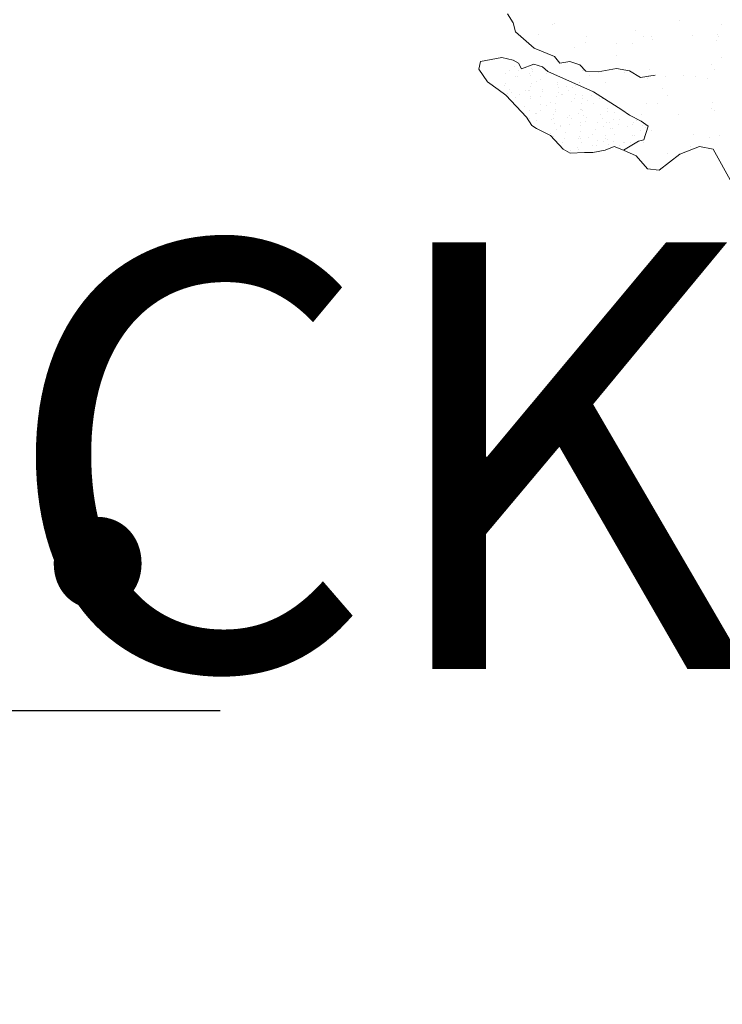
# Model space of a CAD drawing. Units: inches. Extents: x 1986 to 21484, y -1816 to 2016.
# Tile 50 of 85: x 3644.98 to 3656.5, y 1854.64 to 1870.8. Entities that reach past the tile are written whole.
import ezdxf

# ---------------------------------------------------------------- set-up
doc = ezdxf.new("R2010")
doc.units = ezdxf.units.IN
for name, color, linetype, lineweight in [('A-ANNO-DIMS', 2, 'Continuous', 18), ('A-ANNO-TEXT', 7, 'Continuous', 18), ('L-PLNT', 84, 'Continuous', 13)]:
    doc.layers.add(name, color=color, linetype=linetype, lineweight=lineweight)
doc.styles.get("Standard").update_dxf_attribs({"font": 'arial.ttf'})
doc.dimstyles.new('ISO-25', dxfattribs={"dimtxt": 8, "dimasz": 2.5, "dimexe": 1.25, "dimexo": 0.625, "dimtad": 1, "dimdec": 1, "dimlunit": 3, "dimtxsty": 'Standard', "dimcen": 2.5, "dimadec": 0, "dimazin": 0, "dimtfac": 1, "dimtdec": 1, "dimtmove": 0, "dimatfit": 3, "dimfxl": 1, "dimarcsym": 0})

# ---------------------------------------------------------------- blocks, each defined once
blk = doc.blocks.new('PLANT-SHRUB')
for p, q in [((2183.802, 1893.071), (2183.646, 1892.457)), ((2183.414, 1892.368), (2183.414, 1892.368)), ((2183.646, 1892.457), (2183.781, 1892.27)), ((2183.554, 1892.272), (2183.554, 1892.272)), ((2183.781, 1892.27), (2184.104, 1892.145)), ((2183.781, 1892.27), (2183.781, 1892.27)), ((2183.191, 1892.014), (2183.191, 1892.014)), ((2183.719, 1892.055), (2183.719, 1892.055)), ((2183.888, 1892.163), (2183.888, 1892.163)), ((2184.104, 1892.145), (2184.53, 1892.104)), ((2184.53, 1892.104), (2184.655, 1891.958)), ((2183.132, 1891.886), (2183.132, 1891.886)), ((2183.206, 1891.953), (2183.206, 1891.953)), ((2184.237, 1892), (2184.237, 1892)), ((2184.655, 1891.958), (2184.642, 1891.674)), ((2182.927, 1891.551), (2182.927, 1891.551)), ((2183.673, 1891.644), (2183.673, 1891.644)), ((2184.166, 1891.453), (2184.371, 1891.57)), ((2184.172, 1891.548), (2184.172, 1891.548)), ((2184.334, 1891.535), (2184.334, 1891.535)), ((2184.371, 1891.57), (2184.451, 1891.526)), ((2184.407, 1891.602), (2184.407, 1891.602)), ((2184.435, 1891.533), (2184.435, 1891.533)), ((2184.451, 1891.526), (2184.73, 1891.462)), ((2184.642, 1891.674), (2184.73, 1891.462)), ((2182.512, 1891.452), (2182.512, 1891.452)), ((2182.72, 1891.424), (2182.72, 1891.424)), ((2182.734, 1891.521), (2182.734, 1891.521)), ((2183.045, 1891.382), (2183.045, 1891.382)), ((2184.195, 1891.314), (2184.166, 1891.453)), ((2184.217, 1891.434), (2184.217, 1891.434)), ((2184.219, 1891.383), (2184.219, 1891.383)), ((2184.3, 1891.423), (2184.3, 1891.423)), ((2184.43, 1891.406), (2184.43, 1891.406)), ((2184.47, 1891.389), (2184.47, 1891.389)), ((2184.567, 1891.453), (2184.567, 1891.453)), ((2184.628, 1891.385), (2184.628, 1891.385)), ((2184.647, 1891.378), (2184.647, 1891.378)), ((2184.73, 1891.462), (2184.803, 1891.316)), ((2184.731, 1891.367), (2184.731, 1891.367)), ((2183.166, 1891.244), (2183.166, 1891.244)), ((2183.588, 1891.31), (2183.588, 1891.31)), ((2183.796, 1891.283), (2183.796, 1891.283)), ((2184.121, 1891.24), (2184.121, 1891.24)), ((2184.268, 1891.11), (2184.195, 1891.314)), ((2184.212, 1891.23), (2184.212, 1891.23)), ((2184.25, 1891.252), (2184.25, 1891.252)), ((2184.301, 1891.235), (2184.301, 1891.235)), ((2184.33, 1891.262), (2184.33, 1891.262)), ((2184.425, 1891.225), (2184.425, 1891.225)), ((2184.748, 1891.251), (2184.748, 1891.251)), ((2184.803, 1891.316), (2184.949, 1891.258)), ((2184.844, 1891.219), (2184.844, 1891.219)), ((2184.949, 1891.258), (2185.124, 1891.148)), ((2182.152, 1891.057), (2182.152, 1891.057)), ((2182.313, 1891.135), (2182.313, 1891.135)), ((2182.32, 1891.164), (2182.32, 1891.164)), ((2182.387, 1891.202), (2182.387, 1891.202)), ((2183.396, 1891.055), (2183.396, 1891.055)), ((2183.565, 1891.162), (2183.565, 1891.162)), ((2183.936, 1891.17), (2183.936, 1891.17)), ((2184.298, 1890.964), (2184.268, 1891.11)), ((2184.438, 1891.053), (2184.438, 1891.053)), ((2184.506, 1891.096), (2184.506, 1891.096)), ((2184.618, 1891.077), (2184.618, 1891.077)), ((2184.641, 1891.052), (2184.641, 1891.052)), ((2184.664, 1891.169), (2184.664, 1891.169)), ((2184.782, 1891.094), (2184.782, 1891.094)), ((2184.81, 1891.16), (2184.81, 1891.16)), ((2184.811, 1891.121), (2184.811, 1891.121)), ((2184.872, 1891.141), (2184.872, 1891.141)), ((2184.936, 1891.052), (2184.936, 1891.052)), ((2185.003, 1891.095), (2185.003, 1891.095)), ((2185.05, 1891.061), (2185.05, 1891.061)), ((2185.124, 1891.148), (2185.227, 1891.053)), ((2185.227, 1891.053), (2185.402, 1890.9)), ((2183.511, 1890.923), (2183.71, 1890.783)), ((2184.437, 1890.428), (2184.298, 1890.964)), ((2184.415, 1890.917), (2184.415, 1890.917)), ((2184.5, 1890.983), (2184.5, 1890.983)), ((2184.583, 1890.972), (2184.583, 1890.972)), ((2184.622, 1890.948), (2184.622, 1890.948)), ((2184.713, 1890.955), (2184.713, 1890.955)), ((2184.834, 1890.911), (2184.834, 1890.911)), ((2184.93, 1890.927), (2184.93, 1890.927)), ((2185.014, 1890.916), (2185.014, 1890.916)), ((2185.144, 1890.898), (2185.144, 1890.898)), ((2185.242, 1890.913), (2185.242, 1890.913)), ((2185.262, 1890.954), (2185.262, 1890.954)), ((2185.402, 1890.9), (2185.439, 1890.775)), ((2182.625, 1890.869), (2182.625, 1890.869)), ((2183.515, 1890.784), (2183.515, 1890.784)), ((2183.588, 1890.852), (2183.588, 1890.852)), ((2183.648, 1890.874), (2183.648, 1890.874)), ((2183.71, 1890.783), (2183.768, 1890.584)), ((2184.454, 1890.794), (2184.454, 1890.794)), ((2184.483, 1890.821), (2184.483, 1890.821)), ((2184.608, 1890.769), (2184.608, 1890.769)), ((2184.619, 1890.85), (2184.619, 1890.85)), ((2184.727, 1890.835), (2184.727, 1890.835)), ((2185.04, 1890.753), (2185.04, 1890.753)), ((2185.103, 1890.808), (2185.103, 1890.808)), ((2185.117, 1890.849), (2185.117, 1890.849)), ((2185.137, 1890.82), (2185.137, 1890.82)), ((2185.361, 1890.87), (2185.361, 1890.87)), ((2185.439, 1890.775), (2185.439, 1890.468)), ((2183.768, 1890.584), (2183.897, 1890.409)), ((2184.376, 1890.696), (2184.376, 1890.696)), ((2184.405, 1890.609), (2184.405, 1890.609)), ((2184.436, 1890.578), (2184.436, 1890.578)), ((2184.566, 1890.561), (2184.566, 1890.561)), ((2184.807, 1890.652), (2184.807, 1890.652)), ((2184.823, 1890.603), (2184.823, 1890.603)), ((2184.874, 1890.695), (2184.874, 1890.695)), ((2184.934, 1890.654), (2184.934, 1890.654)), ((2184.964, 1890.681), (2184.964, 1890.681)), ((2185.232, 1890.605), (2185.232, 1890.605)), ((2185.305, 1890.651), (2185.305, 1890.651)), ((2185.372, 1890.694), (2185.372, 1890.694)), ((2182.604, 1890.55), (2182.604, 1890.55)), ((2183.117, 1890.42), (2183.117, 1890.42)), ((2183.141, 1890.474), (2183.141, 1890.474)), ((2183.849, 1890.548), (2183.849, 1890.548)), ((2183.897, 1890.409), (2184.154, 1890.245)), ((2184.187, 1890.46), (2184.187, 1890.46)), ((2184.752, 1889.675), (2184.437, 1890.428)), ((2184.49, 1890.45), (2184.49, 1890.45)), ((2184.598, 1890.461), (2184.598, 1890.461)), ((2184.716, 1890.433), (2184.716, 1890.433)), ((2184.775, 1890.508), (2184.775, 1890.508)), ((2184.783, 1890.532), (2184.783, 1890.532)), ((2184.79, 1890.501), (2184.79, 1890.501)), ((2184.866, 1890.521), (2184.866, 1890.521)), ((2184.988, 1890.449), (2184.988, 1890.449)), ((2184.996, 1890.504), (2184.996, 1890.504)), ((2185.03, 1890.445), (2185.03, 1890.445)), ((2185.093, 1890.545), (2185.093, 1890.545)), ((2185.209, 1890.465), (2185.209, 1890.465)), ((2185.213, 1890.475), (2185.213, 1890.475)), ((2185.297, 1890.464), (2185.297, 1890.464)), ((2185.415, 1890.513), (2185.415, 1890.513)), ((2185.426, 1890.447), (2185.426, 1890.447)), ((2185.439, 1890.468), (2185.527, 1890.227)), ((2185.448, 1890.44), (2185.448, 1890.44)), ((2183.22, 1890.324), (2183.22, 1890.324)), ((2183.428, 1890.297), (2183.428, 1890.297)), ((2183.753, 1890.254), (2183.753, 1890.254)), ((2184.154, 1890.245), (2184.294, 1890.093)), ((2184.607, 1890.353), (2184.607, 1890.353)), ((2184.636, 1890.38), (2184.636, 1890.38)), ((2184.678, 1890.252), (2184.678, 1890.252)), ((2184.745, 1890.295), (2184.745, 1890.295)), ((2184.813, 1890.295), (2184.813, 1890.295)), ((2185.117, 1890.24), (2185.117, 1890.24)), ((2185.176, 1890.251), (2185.176, 1890.251)), ((2185.222, 1890.297), (2185.222, 1890.297)), ((2185.243, 1890.294), (2185.243, 1890.294)), ((2185.256, 1890.368), (2185.256, 1890.368)), ((2183.242, 1890.161), (2183.242, 1890.161)), ((2183.623, 1890.104), (2183.623, 1890.104)), ((2184.294, 1890.093), (2184.294, 1889.953)), ((2184.296, 1890.182), (2184.296, 1890.182)), ((2184.487, 1890.159), (2184.487, 1890.159)), ((2184.504, 1890.155), (2184.504, 1890.155)), ((2184.588, 1890.153), (2184.588, 1890.153)), ((2184.636, 1890.138), (2184.636, 1890.138)), ((2184.719, 1890.127), (2184.719, 1890.127)), ((2184.829, 1890.112), (2184.829, 1890.112)), ((2184.849, 1890.109), (2184.849, 1890.109)), ((2185.019, 1890.137), (2185.019, 1890.137)), ((2185.066, 1890.081), (2185.066, 1890.081)), ((2185.087, 1890.213), (2185.087, 1890.213)), ((2185.438, 1890.132), (2185.438, 1890.132)), ((2185.549, 1890.14), (2185.519, 1889.979)), ((2185.527, 1890.227), (2185.549, 1890.14)), ((2184.294, 1889.953), (2184.376, 1889.801)), ((2184.318, 1890.069), (2184.318, 1890.069)), ((2184.318, 1890.051), (2184.318, 1890.051)), ((2184.702, 1890.065), (2184.702, 1890.065)), ((2184.76, 1889.913), (2184.76, 1889.913)), ((2184.789, 1889.94), (2184.789, 1889.94)), ((2184.803, 1889.987), (2184.803, 1889.987)), ((2184.859, 1890.049), (2184.859, 1890.049)), ((2184.928, 1890.067), (2184.928, 1890.067)), ((2185.149, 1890.07), (2185.149, 1890.07)), ((2185.212, 1889.989), (2185.212, 1889.989)), ((2185.279, 1890.053), (2185.279, 1890.053)), ((2185.357, 1890.048), (2185.357, 1890.048)), ((2185.371, 1890.041), (2185.371, 1890.041)), ((2185.409, 1889.927), (2185.409, 1889.927)), ((2185.496, 1890.024), (2185.496, 1890.024)), ((2185.519, 1889.979), (2185.52, 1889.485)), ((2183.97, 1889.75), (2183.97, 1889.75)), ((2184.376, 1889.801), (2184.517, 1889.708)), ((2185.009, 1889.829), (2185.009, 1889.829)), ((2185.046, 1889.85), (2185.046, 1889.85)), ((2185.114, 1889.893), (2185.114, 1889.893)), ((2185.24, 1889.773), (2185.24, 1889.773)), ((2185.27, 1889.8), (2185.27, 1889.8)), ((2185.428, 1889.824), (2185.428, 1889.824)), ((2183.897, 1889.683), (2183.897, 1889.683)), ((2184.162, 1889.69), (2184.162, 1889.69)), ((2184.517, 1889.708), (2184.505, 1889.567)), ((2184.766, 1889.558), (2184.752, 1889.675)), ((2184.793, 1889.679), (2184.793, 1889.679)), ((2184.919, 1889.686), (2184.919, 1889.686)), ((2185.002, 1889.675), (2185.002, 1889.675)), ((2185.081, 1889.627), (2185.081, 1889.627)), ((2185.132, 1889.658), (2185.132, 1889.658)), ((2185.184, 1889.695), (2185.184, 1889.695)), ((2185.202, 1889.681), (2185.202, 1889.681)), ((2185.227, 1889.648), (2185.227, 1889.648)), ((2185.349, 1889.63), (2185.349, 1889.63)), ((2185.432, 1889.619), (2185.432, 1889.619)), ((2184.505, 1889.567), (2184.655, 1889.238)), ((2184.505, 1889.567), (2184.505, 1889.567)), ((2184.839, 1889.427), (2184.766, 1889.558)), ((2185.037, 1889.346), (2184.839, 1889.427)), ((2184.913, 1889.472), (2184.913, 1889.472)), ((2184.917, 1889.45), (2184.917, 1889.45)), ((2184.942, 1889.499), (2184.942, 1889.499)), ((2184.985, 1889.493), (2184.985, 1889.493)), ((2184.999, 1889.521), (2184.999, 1889.521)), ((2185.415, 1889.449), (2185.415, 1889.449)), ((2185.418, 1889.516), (2185.418, 1889.516)), ((2185.483, 1889.492), (2185.483, 1889.492)), ((2185.52, 1889.485), (2185.549, 1889.332)), ((2185.008, 1889.244), (2185.037, 1889.346)), ((2185.098, 1889.332), (2185.098, 1889.332)), ((2185.172, 1889.4), (2185.172, 1889.4)), ((2185.192, 1889.373), (2185.192, 1889.373)), ((2185.393, 1889.332), (2185.393, 1889.332)), ((2185.423, 1889.359), (2185.423, 1889.359)), ((2185.549, 1889.332), (2185.593, 1889.12)), ((2184.135, 1889.169), (2184.135, 1889.169)), ((2184.164, 1889.158), (2184.164, 1889.158)), ((2184.46, 1889.126), (2184.46, 1889.126)), ((2184.655, 1889.238), (2184.696, 1888.836)), ((2184.655, 1889.238), (2184.655, 1889.238)), ((2185.037, 1889.149), (2185.008, 1889.244)), ((2185.147, 1888.988), (2185.037, 1889.149)), ((2185.098, 1889.247), (2185.098, 1889.247)), ((2185.201, 1889.235), (2185.201, 1889.235)), ((2185.285, 1889.224), (2185.285, 1889.224)), ((2185.593, 1889.12), (2185.549, 1888.871)), ((2185.446, 1888.798), (2185.147, 1888.988)), ((2184.696, 1888.836), (2184.622, 1888.704)), ((2185.549, 1888.871), (2185.446, 1888.798)), ((2185.446, 1888.798), (2185.446, 1888.798)), ((2184.622, 1888.704), (2184.589, 1888.532))]:
    blk.add_line(p, q)
blk = doc.blocks.new('*D96')
at = {"layer": 'A-ANNO-DIMS', "color": 0, "lineweight": -2, "transparency": 16777216}
for p, q in [((3539.82, 1864.464), (3539.82, 1858.215)), ((3577.115, 1864.464), (3577.115, 1858.215)), ((3542.32, 1859.465), (3574.615, 1859.465)), ((3577.115, 1859.465), (3648.265, 1859.465))]:
    blk.add_line(p, q, dxfattribs=at)
at = {"layer": 'A-ANNO-DIMS', "color": 0, "transparency": 16777216}
for points in [[(3542.32, 1859.882), (3542.32, 1859.048), (3539.82, 1859.465)], [(3574.615, 1859.882), (3574.615, 1859.048), (3577.115, 1859.465)]]:
    blk.add_solid(points, dxfattribs=at)
at = {"layer": 'Defpoints', "color": 0, "transparency": 16777216}
for p in [(3539.82, 1865.089), (3577.115, 1865.089), (3577.115, 1859.465)]:
    blk.add_point(p, dxfattribs=at)
at = {"layer": 'A-ANNO-DIMS', "color": 0, "transparency": 16777216, "insert": (3613.94, 1864.229), "char_height": 8, "attachment_point": 5}
blk.add_mtext('3\'-1 1/2" TYP.', dxfattribs=at)

msp = doc.modelspace()

# ---------------------------------------------------------------- block references
at = {"layer": 'L-PLNT', "rotation": 223.1883365522388}
msp.add_blockref('PLANT-SHRUB', (3953.27, 4742.965), dxfattribs=at)

# ---------------------------------------------------------------- texts
at = {"layer": 'A-ANNO-TEXT', "insert": (3605.478, 1867.143), "char_height": 7, "attachment_point": 1}
msp.add_mtext_dynamic_manual_height_columns("{\\fTimes New Roman|b0|i0|c0|p18;4' SETBACK}", width=105.61268, gutter_width=12.5, heights=[0], dxfattribs=at)

# ---------------------------------------------------------------- dimensions: what is measured, and where the dimension line sits
at = {"layer": 'A-ANNO-DIMS'}
dim = msp.add_linear_dim(base=(3577.115, 1859.465), p1=(3539.82, 1865.089), p2=(3577.115, 1865.089), text='<> TYP.', dimstyle='ISO-25', override={"dimdec": 1, "dimrnd": 0, "dimzin": 1, "dimlunit": 4, "dimfrac": 2}, dxfattribs=at)
dim.commit()
dim.dimension.update_dxf_attribs({"geometry": '*D96', "text_midpoint": (3613.94, 1864.229)})

doc.saveas('drawing.dxf')
